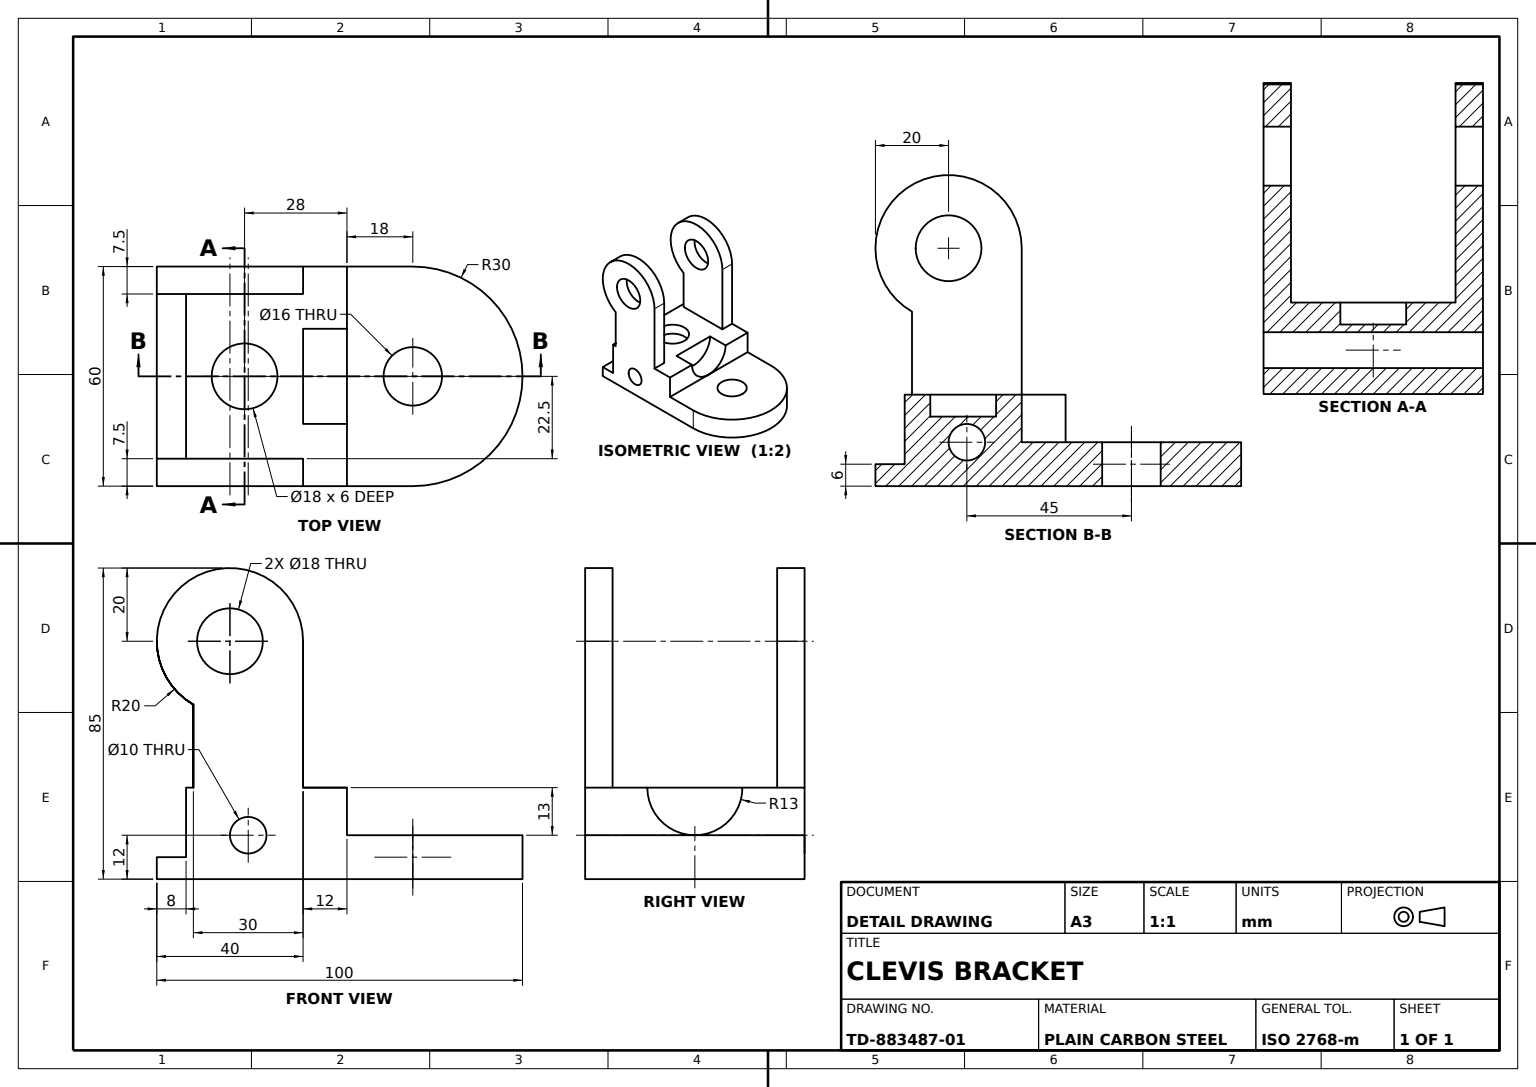
from build123d import *

# Parameters (mm, degrees)
BASE_PLATE_DEPTH         = 12
CENTRE_HOLE_16_SKETCH_R  = 8
CENTRE_HOLE_16_DEPTH     = 12
GROOVE_SKETCH_W          = 60
GROOVE_SKETCH_H          = 8
GROOVE_8MM_DEPTH         = 6
UPRIGHT_WALL_DEPTH       = 60
PIN_LUG_SKETCH_R         = 9
PIN_LUG_DEPTH            = 7.5
HOLE_26_SKETCH_R         = 13
HOLE_26_DEPTH            = 12
RECESS_18_SKETCH_R       = 9
RECESS_18_DEPTH          = 6
SIDE_HOLE_10_SKETCH_R    = 5
SIDE_HOLE_10_DEPTH       = 13
LUG_START                = -85
LUG_PIN_HOLE_10_SKETCH_R = 5
LUG_PIN_HOLE_10_DEPTH    = 85


with BuildPart() as part:
    # Base Plate Sketch → Base Plate (new body)
    with BuildSketch(Plane(origin=(0, 0, 0), x_dir=(1, 0, 0), z_dir=(0, 1, 0))):
        with BuildLine():
            Line((30, 0), (30, -70))
            Line((30, -70), (-30, -70))
            Line((-30, -70), (-30, 0))
            ThreePointArc((-30, 0), (0, 30), (30, 0))
        make_face()
    extrude(amount=BASE_PLATE_DEPTH)

    # Centre Hole Ø16 Sketch → Centre Hole Ø16 (cut)
    with BuildSketch(Plane(origin=(0, 12, 0), x_dir=(1, 0, 0), z_dir=(0, 1, 0))):
        with Locations(Location((0, 0, 0), (0, 0, 270))):
            Circle(CENTRE_HOLE_16_SKETCH_R)
    extrude(amount=-CENTRE_HOLE_16_DEPTH, mode=Mode.SUBTRACT)

    # Groove Sketch → Groove 8mm (cut)
    with BuildSketch(Plane(origin=(0, 12, 0), x_dir=(1, 0, 0), z_dir=(0, 1, 0))):
        with Locations((0, -66)):
            Rectangle(GROOVE_SKETCH_W, GROOVE_SKETCH_H)
    extrude(amount=-GROOVE_8MM_DEPTH, mode=Mode.SUBTRACT)

    # Upright Wall Sketch → Upright Wall (add)
    with BuildSketch(Plane(origin=(30, 0, 0), x_dir=(0, 0, -1), z_dir=(1, 0, 0))):
        Polygon((-62, 12), (-18, 12), (-18, 25), (-30, 25), (-62, 25), align=None)
    extrude(amount=-UPRIGHT_WALL_DEPTH)

    # Pin Lug Sketch → Pin Lug (add)
    with BuildSketch(Plane(origin=(30, 0, 0), x_dir=(0, 0, -1), z_dir=(1, 0, 0))):
        with BuildLine():
            Line((-60, 25), (-30, 25))
            Line((-30, 25), (-30, 65))
            ThreePointArc((-30, 65), (-60, 82.320508076), (-60, 47.679491924))
            Line((-60, 47.679491924), (-60, 25))
        make_face()
        with Locations((-50, 65)):
            Circle(PIN_LUG_SKETCH_R, mode=Mode.SUBTRACT)
    pin_lug = extrude(amount=-PIN_LUG_DEPTH)

    # Pin Lug Mirror: Pin Lug across plane
    add(pin_lug.mirror(Plane(origin=(0, 0, 0), x_dir=(0, 0, 1), z_dir=(1, 0, 0))))

    # Hole Ø26 Sketch → Hole Ø26 (cut)
    with BuildSketch(Plane(origin=(0, 0, 18), x_dir=(-1, 0, 0), z_dir=(0, 0, -1))):
        with Locations((0, 25)):
            Circle(HOLE_26_SKETCH_R)
    extrude(amount=-HOLE_26_DEPTH, mode=Mode.SUBTRACT)

    # Recess Ø18 Sketch → Recess Ø18 (cut)
    with BuildSketch(Plane(origin=(0, 25, 0), x_dir=(1, 0, 0), z_dir=(0, 1, 0))):
        with Locations(Location((0, -46, 0), (0, 0, 270))):
            Circle(RECESS_18_SKETCH_R)
    extrude(amount=-RECESS_18_DEPTH, mode=Mode.SUBTRACT)

    # Side Hole Ø10 Sketch → Side Hole Ø10 (cut)
    with BuildSketch(Plane(origin=(30, 0, 0), x_dir=(0, 0, -1), z_dir=(1, 0, 0))):
        with Locations((-45, 12)):
            Circle(SIDE_HOLE_10_SKETCH_R)
    extrude(amount=-SIDE_HOLE_10_DEPTH, mode=Mode.SUBTRACT)

    # Lug Pin Hole Ø10 Sketch → Lug Pin Hole Ø10 (cut)
    with BuildSketch(Plane.ZY.offset(30).offset(LUG_START)):
        with Locations(Location((45, 12, 0), (0, 0, 180))):
            Circle(LUG_PIN_HOLE_10_SKETCH_R)
    extrude(amount=LUG_PIN_HOLE_10_DEPTH, mode=Mode.SUBTRACT)


solid = part.part
